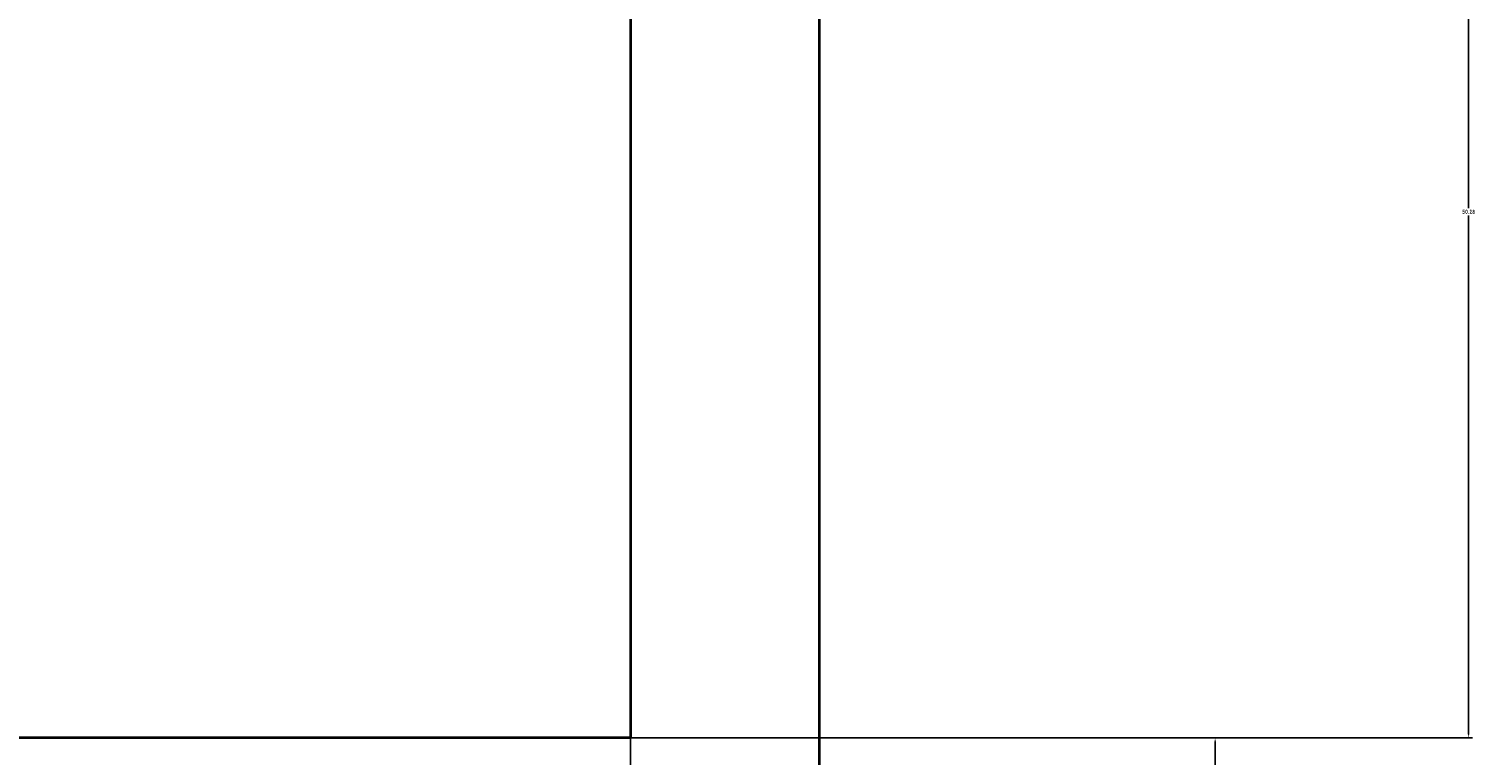
# Model space of a CAD drawing. Units: feet. Extents: x 1654 to 2985, y 1348 to 2230.
# Tile 37 of 53: x 2173 to 2242, y 1750 to 1785. Entities that reach past the tile are written whole.
import ezdxf

# ---------------------------------------------------------------- set-up
doc = ezdxf.new("R2010")
doc.units = ezdxf.units.FT
doc.layers.add('A-ANNO-DIMS', color=2, linetype='Continuous', lineweight=18)
doc.layers.add('A-WALL', color=7, linetype='Continuous', lineweight=35)
doc.styles.get("Standard").update_dxf_attribs({"font": 'arial.ttf'})
doc.dimstyles.get("Standard").update_dxf_attribs({"dimtxt": 0.18, "dimasz": 0.18, "dimexe": 0.18, "dimexo": 0.0625, "dimgap": 0.09, "dimtad": 0, "dimtih": 1, "dimtoh": 1, "dimdec": 4, "dimzin": 0, "dimdsep": 46, "dimtxsty": 'Standard', "dimcen": 0.09, "dimadec": 0, "dimazin": 0, "dimtfac": 1, "dimtdec": 4, "dimtofl": 0, "dimtmove": 0, "dimatfit": 3, "dimfxl": 1, "dimtolj": 1, "dimtzin": 0, "dimarcsym": 0})

# ---------------------------------------------------------------- blocks, each defined once
blk = doc.blocks.new('*D72')
at = {"layer": 'A-ANNO-DIMS', "color": 0, "lineweight": -2, "transparency": 16777216}
for p, q in [((2202.155, 1751.255), (2230.172, 1751.255)), ((2229.992, 1751.075), (2229.992, 1658.438)), ((2229.992, 1565.435), (2229.992, 1658.072)), ((2202.155, 1565.255), (2230.172, 1565.255))]:
    blk.add_line(p, q, dxfattribs=at)
at = {"layer": 'A-ANNO-DIMS', "color": 0, "transparency": 16777216}
for points in [[(2229.962, 1751.075), (2230.022, 1751.075), (2229.992, 1751.255)], [(2229.962, 1565.435), (2230.022, 1565.435), (2229.992, 1565.255)]]:
    blk.add_solid(points, dxfattribs=at)
at = {"layer": 'Defpoints', "color": 0, "transparency": 16777216}
for p in [(2202.092, 1751.255), (2229.992, 1751.255), (2202.092, 1565.255)]:
    blk.add_point(p, dxfattribs=at)
at = {"layer": 'A-ANNO-DIMS', "color": 0, "transparency": 16777216, "insert": (2229.992, 1658.255), "char_height": 0.18, "attachment_point": 5}
blk.add_mtext('\\A1;STAIR 186 TYP.', dxfattribs=at)
blk = doc.blocks.new('*D80')
at = {"layer": 'A-ANNO-DIMS', "color": 0, "lineweight": -2, "transparency": 16777216}
for p, q in [((2070.092, 2039.192), (2070.092, 1534.075)), ((2202.092, 2039.192), (2202.092, 1534.075)), ((2070.272, 1534.255), (2135.813, 1534.255)), ((2201.912, 1534.255), (2136.372, 1534.255))]:
    blk.add_line(p, q, dxfattribs=at)
at = {"layer": 'A-ANNO-DIMS', "color": 0, "transparency": 16777216}
for points in [[(2070.272, 1534.285), (2070.272, 1534.225), (2070.092, 1534.255)], [(2201.912, 1534.285), (2201.912, 1534.225), (2202.092, 1534.255)]]:
    blk.add_solid(points, dxfattribs=at)
at = {"layer": 'Defpoints', "color": 0, "transparency": 16777216}
for p in [(2070.092, 2039.255), (2202.092, 2039.255), (2202.092, 1534.255)]:
    blk.add_point(p, dxfattribs=at)
at = {"layer": 'A-ANNO-DIMS', "color": 0, "transparency": 16777216, "insert": (2136.092, 1534.255), "char_height": 0.18, "attachment_point": 5}
blk.add_mtext('\\A1;132', dxfattribs=at)
blk = doc.blocks.new('*D91')
at = {"layer": 'A-ANNO-DIMS', "color": 0, "lineweight": -2, "transparency": 16777216}
for p, q in [((1852.155, 1801.468), (2242.272, 1801.468)), ((2242.092, 1801.288), (2242.092, 1776.544)), ((2242.092, 1751.435), (2242.092, 1776.18)), ((1852.155, 1751.255), (2242.272, 1751.255))]:
    blk.add_line(p, q, dxfattribs=at)
at = {"layer": 'A-ANNO-DIMS', "color": 0, "transparency": 16777216}
for points in [[(2242.062, 1801.288), (2242.122, 1801.288), (2242.092, 1801.468)], [(2242.062, 1751.435), (2242.122, 1751.435), (2242.092, 1751.255)]]:
    blk.add_solid(points, dxfattribs=at)
at = {"layer": 'Defpoints', "color": 0, "transparency": 16777216}
for p in [(1852.092, 1801.468), (2242.092, 1801.468), (1852.092, 1751.255)]:
    blk.add_point(p, dxfattribs=at)
at = {"layer": 'A-ANNO-DIMS', "color": 0, "transparency": 16777216, "insert": (2242.092, 1776.362), "char_height": 0.18, "attachment_point": 5}
blk.add_mtext('\\A1;50.21', dxfattribs=at)
blk = doc.blocks.new('*D96')
at = {"layer": 'A-ANNO-DIMS', "color": 0, "lineweight": -2, "transparency": 16777216}
for p, q in [((2202.155, 1801.437), (2242.272, 1801.437)), ((2242.092, 1801.257), (2242.092, 1776.528)), ((2242.092, 1751.435), (2242.092, 1776.164)), ((2202.155, 1751.255), (2242.272, 1751.255))]:
    blk.add_line(p, q, dxfattribs=at)
at = {"layer": 'A-ANNO-DIMS', "color": 0, "transparency": 16777216}
for points in [[(2242.062, 1801.257), (2242.122, 1801.257), (2242.092, 1801.437)], [(2242.062, 1751.435), (2242.122, 1751.435), (2242.092, 1751.255)]]:
    blk.add_solid(points, dxfattribs=at)
at = {"layer": 'Defpoints', "color": 0, "transparency": 16777216}
for p in [(2202.092, 1801.437), (2242.092, 1801.437), (2202.092, 1751.255)]:
    blk.add_point(p, dxfattribs=at)
at = {"layer": 'A-ANNO-DIMS', "color": 0, "transparency": 16777216, "insert": (2242.092, 1776.346), "char_height": 0.18, "attachment_point": 5}
blk.add_mtext('\\A1;50.18', dxfattribs=at)

msp = doc.modelspace()

# ---------------------------------------------------------------- linework, layer by layer
at = {"layer": 'A-WALL'}
for p, q in [((2211.0924, 2117.2549), (2211.0924, 1742.2549)), ((2202.0924, 1886.2549), (2202.0924, 1751.2549)), ((2211.0924, 1886.2549), (2211.0924, 1565.2549)), ((2202.0924, 1751.2549), (2120.0924, 1751.2549))]:
    msp.add_line(p, q, dxfattribs=at)

# ---------------------------------------------------------------- dimensions: what is measured, and where the dimension line sits
at = {"layer": 'A-ANNO-DIMS'}
dim = msp.add_linear_dim(base=(2202.0924, 1534.2549), p1=(2070.0924, 2039.2549), p2=(2202.0924, 2039.2549), dimstyle='Standard', override={"dimdec": 0, "dimlfac": 1, "dimrnd": 0, "dimzin": 0, "dimdsep": 46, "dimlunit": 2}, dxfattribs=at)
dim.commit()
dim.dimension.update_dxf_attribs({"geometry": '*D80', "text_midpoint": (2136.0924, 1534.2549)})
for base, p1, p2, picture, middle in [((2242.0924, 1801.4683), (1852.0924, 1751.2549), (1852.0924, 1801.4683), '*D91', (2242.0924, 1776.3616)), ((2242.0924, 1801.4371), (2202.0924, 1751.2549), (2202.0924, 1801.4371), '*D96', (2242.0924, 1776.346))]:
    dim = msp.add_linear_dim(base=base, p1=p1, p2=p2, angle=90, dimstyle='Standard', override={"dimdec": 2, "dimlfac": 1, "dimrnd": 0, "dimzin": 0, "dimdsep": 46, "dimlunit": 2}, dxfattribs=at)
    dim.commit()
    dim.dimension.update_dxf_attribs({"geometry": picture, "text_midpoint": middle})
dim = msp.add_linear_dim(base=(2229.9924, 1751.2549), p1=(2202.0924, 1565.2549), p2=(2202.0924, 1751.2549), angle=90, text='STAIR <> TYP.', dimstyle='Standard', override={"dimdec": 0, "dimlfac": 1, "dimrnd": 0, "dimzin": 0, "dimdsep": 46, "dimlunit": 2}, dxfattribs=at)
dim.commit()
dim.dimension.update_dxf_attribs({"geometry": '*D72', "text_midpoint": (2229.9924, 1658.2549)})

doc.saveas('drawing.dxf')
